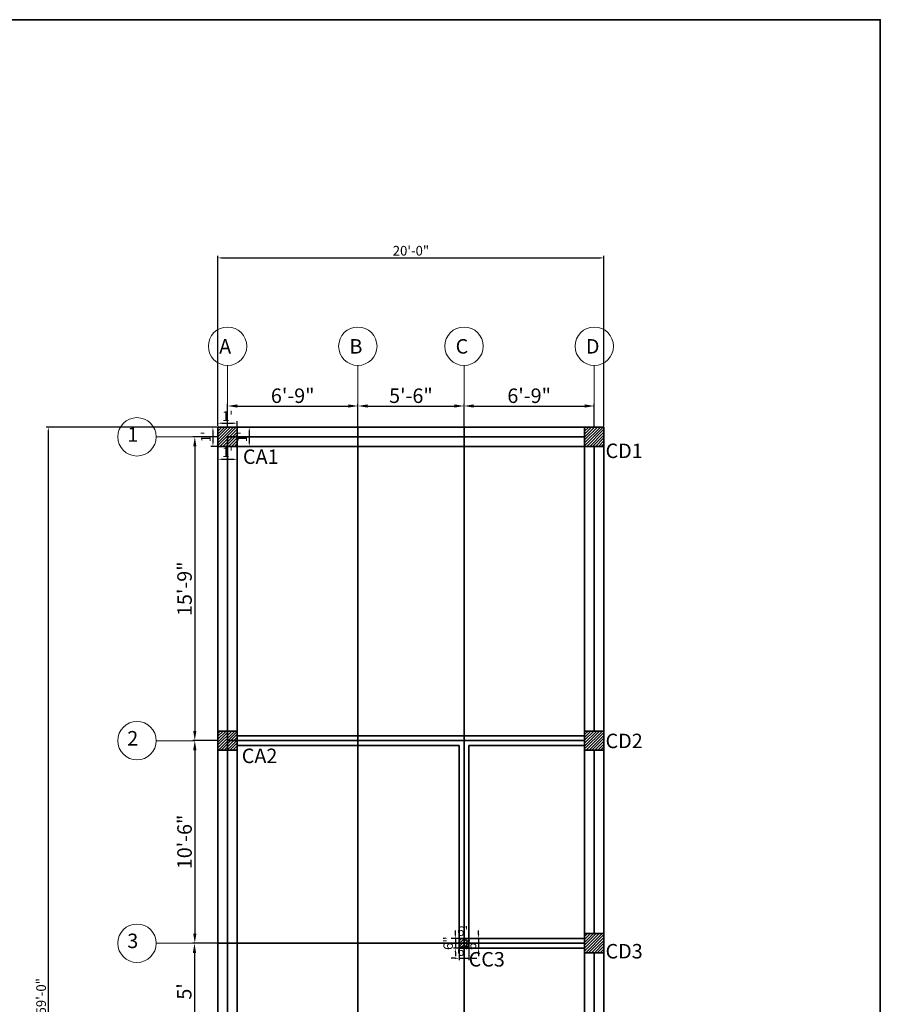
# Model space of a CAD drawing. Units: millimetres. Extents: x 20768 to 23556, y 50760 to 52704.
# Tile 36 of 36: x 23021 to 23556, y 52092 to 52704. Entities that reach past the tile are written whole.
import ezdxf

# ---------------------------------------------------------------- set-up
doc = ezdxf.new("R2010")
doc.units = ezdxf.units.MM
for name, color, linetype, lineweight in [('A-ANNO-TTLB', 7, 'Continuous', 35), ('S-ANNO-DIMS', 2, 'Continuous', 18), ('S-ANNO-TEXT', 6, 'Continuous', 18), ('S-BEAM', 3, 'Continuous', 35), ('S-COLS', 20, 'Continuous', 35), ('S-COLS-PATT', 8, 'Continuous', 13), ('S-GRID', 1, 'Continuous', 18)]:
    doc.layers.add(name, color=color, linetype=linetype, lineweight=lineweight)
doc.styles.get("Standard").update_dxf_attribs({"font": 'arial.ttf'})
doc.dimstyles.new('ISO-25', dxfattribs={"dimtxt": 6, "dimasz": 2.5, "dimexe": 1.25, "dimexo": 0.625, "dimtad": 1, "dimdec": 0, "dimlunit": 3, "dimtxsty": 'Standard', "dimcen": 2.5, "dimadec": 0, "dimazin": 0, "dimtfac": 1, "dimtdec": 0, "dimtmove": 0, "dimatfit": 3, "dimfxl": 1, "dimarcsym": 0})
pattern_1 = [(45, (1088.7427, 0), (-0.898025612, 0.898025612), [])]

# ---------------------------------------------------------------- blocks, each defined once
blk = doc.blocks.new('*D80')
at = {"layer": 'Defpoints', "color": 0, "transparency": 16777216}
for p in [(23231.01, 52463.68), (23150.01, 52450.51), (23231.01, 52450.51)]:
    blk.add_point(p, dxfattribs=at)
at = {"layer": 'S-ANNO-DIMS', "color": 0, "lineweight": -2, "transparency": 16777216}
for p, q in [((23150.01, 52451.13), (23150.01, 52464.93)), ((23231.01, 52451.13), (23231.01, 52464.93)), ((23156.01, 52463.68), (23225.01, 52463.68))]:
    blk.add_line(p, q, dxfattribs=at)
at = {"layer": 'S-ANNO-DIMS', "color": 0, "transparency": 16777216}
for points in [[(23156.01, 52464.68), (23156.01, 52462.68), (23150.01, 52463.68)], [(23225.01, 52464.68), (23225.01, 52462.68), (23231.01, 52463.68)]]:
    blk.add_solid(points, dxfattribs=at)
at = {"layer": 'S-ANNO-DIMS', "color": 0, "transparency": 16777216, "insert": (23190.51, 52468.9), "char_height": 9, "attachment_point": 5}
blk.add_mtext('6\'-9"', dxfattribs=at)
blk = doc.blocks.new('*D81')
at = {"layer": 'Defpoints', "color": 0, "transparency": 16777216}
for p in [(23297.01, 52463.68), (23231.01, 52450.51), (23297.01, 52450.51)]:
    blk.add_point(p, dxfattribs=at)
at = {"layer": 'S-ANNO-DIMS', "color": 0, "lineweight": -2, "transparency": 16777216}
for p, q in [((23231.01, 52451.13), (23231.01, 52464.93)), ((23297.01, 52451.13), (23297.01, 52464.93)), ((23237.01, 52463.68), (23291.01, 52463.68))]:
    blk.add_line(p, q, dxfattribs=at)
at = {"layer": 'S-ANNO-DIMS', "color": 0, "transparency": 16777216}
for points in [[(23237.01, 52464.68), (23237.01, 52462.68), (23231.01, 52463.68)], [(23291.01, 52464.68), (23291.01, 52462.68), (23297.01, 52463.68)]]:
    blk.add_solid(points, dxfattribs=at)
at = {"layer": 'S-ANNO-DIMS', "color": 0, "transparency": 16777216, "insert": (23264.01, 52468.9), "char_height": 9, "attachment_point": 5}
blk.add_mtext('5\'-6"', dxfattribs=at)
blk = doc.blocks.new('*D82')
at = {"layer": 'Defpoints', "color": 0, "transparency": 16777216}
for p in [(23378.01, 52463.68), (23297.01, 52450.51), (23378.01, 52450.51)]:
    blk.add_point(p, dxfattribs=at)
at = {"layer": 'S-ANNO-DIMS', "color": 0, "lineweight": -2, "transparency": 16777216}
for p, q in [((23297.01, 52451.13), (23297.01, 52464.93)), ((23378.01, 52451.13), (23378.01, 52464.93)), ((23303.01, 52463.68), (23372.01, 52463.68))]:
    blk.add_line(p, q, dxfattribs=at)
at = {"layer": 'S-ANNO-DIMS', "color": 0, "transparency": 16777216}
for points in [[(23303.01, 52464.68), (23303.01, 52462.68), (23297.01, 52463.68)], [(23372.01, 52464.68), (23372.01, 52462.68), (23378.01, 52463.68)]]:
    blk.add_solid(points, dxfattribs=at)
at = {"layer": 'S-ANNO-DIMS', "color": 0, "transparency": 16777216, "insert": (23337.51, 52468.9), "char_height": 9, "attachment_point": 5}
blk.add_mtext('6\'-9"', dxfattribs=at)
blk = doc.blocks.new('*D83')
at = {"layer": 'Defpoints', "color": 0, "transparency": 16777216}
for p in [(23144.01, 52444.51), (23129.65, 52255.51), (23144.01, 52255.51)]:
    blk.add_point(p, dxfattribs=at)
at = {"layer": 'S-ANNO-DIMS', "color": 0, "lineweight": -2, "transparency": 16777216}
for p, q in [((23143.39, 52444.51), (23128.4, 52444.51)), ((23129.65, 52438.51), (23129.65, 52261.51)), ((23143.39, 52255.51), (23128.4, 52255.51))]:
    blk.add_line(p, q, dxfattribs=at)
at = {"layer": 'S-ANNO-DIMS', "color": 0, "transparency": 16777216}
for points in [[(23128.65, 52438.51), (23130.65, 52438.51), (23129.65, 52444.51)], [(23128.65, 52261.51), (23130.65, 52261.51), (23129.65, 52255.51)]]:
    blk.add_solid(points, dxfattribs=at)
at = {"layer": 'S-ANNO-DIMS', "color": 0, "transparency": 16777216, "insert": (23124.43, 52350.01), "char_height": 9, "attachment_point": 5, "rotation": 90}
blk.add_mtext('15\'-9"', dxfattribs=at)
blk = doc.blocks.new('*D84')
at = {"layer": 'Defpoints', "color": 0, "transparency": 16777216}
for p in [(23144.01, 52255.51), (23129.65, 52129.51), (23144.01, 52129.51)]:
    blk.add_point(p, dxfattribs=at)
at = {"layer": 'S-ANNO-DIMS', "color": 0, "lineweight": -2, "transparency": 16777216}
for p, q in [((23143.39, 52255.51), (23128.4, 52255.51)), ((23129.65, 52249.51), (23129.65, 52135.51)), ((23143.39, 52129.51), (23128.4, 52129.51))]:
    blk.add_line(p, q, dxfattribs=at)
at = {"layer": 'S-ANNO-DIMS', "color": 0, "transparency": 16777216}
for points in [[(23128.65, 52249.51), (23130.65, 52249.51), (23129.65, 52255.51)], [(23128.65, 52135.51), (23130.65, 52135.51), (23129.65, 52129.51)]]:
    blk.add_solid(points, dxfattribs=at)
at = {"layer": 'S-ANNO-DIMS', "color": 0, "transparency": 16777216, "insert": (23124.43, 52192.51), "char_height": 9, "attachment_point": 5, "rotation": 90}
blk.add_mtext('10\'-6"', dxfattribs=at)
blk = doc.blocks.new('*D85')
at = {"layer": 'Defpoints', "color": 0, "transparency": 16777216}
for p in [(23144.01, 52129.51), (23129.44, 52069.51), (23144.01, 52069.51)]:
    blk.add_point(p, dxfattribs=at)
at = {"layer": 'S-ANNO-DIMS', "color": 0, "lineweight": -2, "transparency": 16777216}
for p, q in [((23143.39, 52129.51), (23128.19, 52129.51)), ((23129.44, 52123.51), (23129.44, 52075.51)), ((23143.39, 52069.51), (23128.19, 52069.51))]:
    blk.add_line(p, q, dxfattribs=at)
at = {"layer": 'S-ANNO-DIMS', "color": 0, "transparency": 16777216}
for points in [[(23128.44, 52123.51), (23130.44, 52123.51), (23129.44, 52129.51)], [(23128.44, 52075.51), (23130.44, 52075.51), (23129.44, 52069.51)]]:
    blk.add_solid(points, dxfattribs=at)
at = {"layer": 'S-ANNO-DIMS', "color": 0, "transparency": 16777216, "insert": (23124.24, 52099.51), "char_height": 9, "attachment_point": 5, "rotation": 90}
blk.add_mtext("5'", dxfattribs=at)
blk = doc.blocks.new('*D89')
at = {"layer": 'Defpoints', "color": 0, "transparency": 16777216}
for p in [(23156.01, 52452.99), (23144.01, 52450.51), (23156.01, 52450.51)]:
    blk.add_point(p, dxfattribs=at)
at = {"layer": 'S-ANNO-DIMS', "color": 0, "lineweight": -2, "transparency": 16777216}
for p, q in [((23144.01, 52451.13), (23144.01, 52454.24)), ((23146.51, 52452.99), (23153.51, 52452.99)), ((23156.01, 52451.13), (23156.01, 52454.24))]:
    blk.add_line(p, q, dxfattribs=at)
at = {"layer": 'S-ANNO-DIMS', "color": 0, "transparency": 16777216}
for points in [[(23146.51, 52453.41), (23146.51, 52452.58), (23144.01, 52452.99)], [(23153.51, 52453.41), (23153.51, 52452.58), (23156.01, 52452.99)]]:
    blk.add_solid(points, dxfattribs=at)
at = {"layer": 'S-ANNO-DIMS', "color": 0, "transparency": 16777216, "insert": (23150.01, 52456.63), "char_height": 6, "attachment_point": 5}
blk.add_mtext("1'", dxfattribs=at)
blk = doc.blocks.new('*D90')
at = {"layer": 'Defpoints', "color": 0, "transparency": 16777216}
for p in [(23156.01, 52450.51), (23156.01, 52438.51), (23163.48, 52438.51)]:
    blk.add_point(p, dxfattribs=at)
at = {"layer": 'S-ANNO-DIMS', "color": 0, "lineweight": -2, "transparency": 16777216}
for p, q in [((23156.64, 52450.51), (23164.73, 52450.51)), ((23163.48, 52448.01), (23163.48, 52441.01)), ((23156.64, 52438.51), (23164.73, 52438.51))]:
    blk.add_line(p, q, dxfattribs=at)
at = {"layer": 'S-ANNO-DIMS', "color": 0, "transparency": 16777216}
for points in [[(23163.07, 52448.01), (23163.9, 52448.01), (23163.48, 52450.51)], [(23163.07, 52441.01), (23163.9, 52441.01), (23163.48, 52438.51)]]:
    blk.add_solid(points, dxfattribs=at)
at = {"layer": 'S-ANNO-DIMS', "color": 0, "transparency": 16777216, "insert": (23159.85, 52444.51), "char_height": 6, "attachment_point": 5, "rotation": 90}
blk.add_mtext("1'", dxfattribs=at)
blk = doc.blocks.new('*D91')
at = {"layer": 'Defpoints', "color": 0, "transparency": 16777216}
for p in [(23144.01, 52438.51), (23156.01, 52438.51), (23156.01, 52430.53)]:
    blk.add_point(p, dxfattribs=at)
at = {"layer": 'S-ANNO-DIMS', "color": 0, "lineweight": -2, "transparency": 16777216}
for p, q in [((23144.01, 52437.88), (23144.01, 52429.28)), ((23156.01, 52437.88), (23156.01, 52429.28)), ((23146.51, 52430.53), (23153.51, 52430.53))]:
    blk.add_line(p, q, dxfattribs=at)
at = {"layer": 'S-ANNO-DIMS', "color": 0, "transparency": 16777216}
for points in [[(23146.51, 52430.95), (23146.51, 52430.12), (23144.01, 52430.53)], [(23153.51, 52430.95), (23153.51, 52430.12), (23156.01, 52430.53)]]:
    blk.add_solid(points, dxfattribs=at)
at = {"layer": 'S-ANNO-DIMS', "color": 0, "transparency": 16777216, "insert": (23150.01, 52434.17), "char_height": 6, "attachment_point": 5}
blk.add_mtext("1'", dxfattribs=at)
blk = doc.blocks.new('*D79')
at = {"layer": 'Defpoints', "color": 0, "transparency": 16777216}
for p in [(23144.01, 52450.51), (23140.92, 52438.51), (23144.01, 52438.51)]:
    blk.add_point(p, dxfattribs=at)
at = {"layer": 'S-ANNO-DIMS', "color": 0, "lineweight": -2, "transparency": 16777216}
for p, q in [((23143.39, 52450.51), (23139.67, 52450.51)), ((23140.92, 52448.01), (23140.92, 52441.01)), ((23143.39, 52438.51), (23139.67, 52438.51))]:
    blk.add_line(p, q, dxfattribs=at)
at = {"layer": 'S-ANNO-DIMS', "color": 0, "transparency": 16777216}
for points in [[(23140.51, 52448.01), (23141.34, 52448.01), (23140.92, 52450.51)], [(23140.51, 52441.01), (23141.34, 52441.01), (23140.92, 52438.51)]]:
    blk.add_solid(points, dxfattribs=at)
at = {"layer": 'S-ANNO-DIMS', "color": 0, "transparency": 16777216, "insert": (23137.29, 52444.51), "char_height": 6, "attachment_point": 5, "rotation": 90}
blk.add_mtext("1'", dxfattribs=at)
blk = doc.blocks.new('*D92')
at = {"layer": 'Defpoints', "color": 0, "transparency": 16777216}
for p in [(23294.01, 52132.51), (23300.01, 52132.51), (23300.01, 52132.51)]:
    blk.add_point(p, dxfattribs=at)
at = {"layer": 'S-ANNO-DIMS', "color": 0, "lineweight": -2, "transparency": 16777216}
for p, q in [((23291.51, 52132.51), (23289.01, 52132.51)), ((23294.01, 52133.13), (23294.01, 52133.76)), ((23294.01, 52132.51), (23300.01, 52132.51)), ((23300.01, 52133.13), (23300.01, 52133.76)), ((23302.51, 52132.51), (23305.01, 52132.51))]:
    blk.add_line(p, q, dxfattribs=at)
at = {"layer": 'S-ANNO-DIMS', "color": 0, "transparency": 16777216}
for points in [[(23291.51, 52132.93), (23291.51, 52132.09), (23294.01, 52132.51)], [(23302.51, 52132.93), (23302.51, 52132.09), (23300.01, 52132.51)]]:
    blk.add_solid(points, dxfattribs=at)
at = {"layer": 'S-ANNO-DIMS', "color": 0, "transparency": 16777216, "insert": (23297.01, 52136.2), "char_height": 6, "attachment_point": 5}
blk.add_mtext('6"', dxfattribs=at)
blk = doc.blocks.new('*D93')
at = {"layer": 'Defpoints', "color": 0, "transparency": 16777216}
for p in [(23300.01, 52132.51), (23300.01, 52126.51), (23306.09, 52126.51)]:
    blk.add_point(p, dxfattribs=at)
at = {"layer": 'S-ANNO-DIMS', "color": 0, "lineweight": -2, "transparency": 16777216}
for p, q in [((23306.09, 52135.01), (23306.09, 52137.51)), ((23300.64, 52132.51), (23307.34, 52132.51)), ((23306.09, 52132.51), (23306.09, 52126.51)), ((23300.64, 52126.51), (23307.34, 52126.51)), ((23306.09, 52124.01), (23306.09, 52121.51))]:
    blk.add_line(p, q, dxfattribs=at)
at = {"layer": 'S-ANNO-DIMS', "color": 0, "transparency": 16777216}
for points in [[(23305.67, 52135.01), (23306.5, 52135.01), (23306.09, 52132.51)], [(23305.67, 52124.01), (23306.5, 52124.01), (23306.09, 52126.51)]]:
    blk.add_solid(points, dxfattribs=at)
at = {"layer": 'S-ANNO-DIMS', "color": 0, "transparency": 16777216, "insert": (23302.4, 52129.51), "char_height": 6, "attachment_point": 5, "rotation": 90}
blk.add_mtext('6"', dxfattribs=at)
blk = doc.blocks.new('*D94')
at = {"layer": 'Defpoints', "color": 0, "transparency": 16777216}
for p in [(23294.01, 52126.51), (23300.01, 52126.51), (23300.01, 52120.11)]:
    blk.add_point(p, dxfattribs=at)
at = {"layer": 'S-ANNO-DIMS', "color": 0, "lineweight": -2, "transparency": 16777216}
for p, q in [((23294.01, 52125.88), (23294.01, 52118.86)), ((23300.01, 52125.88), (23300.01, 52118.86)), ((23291.51, 52120.11), (23289.01, 52120.11)), ((23294.01, 52120.11), (23300.01, 52120.11)), ((23302.51, 52120.11), (23305.01, 52120.11))]:
    blk.add_line(p, q, dxfattribs=at)
at = {"layer": 'S-ANNO-DIMS', "color": 0, "transparency": 16777216}
for points in [[(23291.51, 52120.52), (23291.51, 52119.69), (23294.01, 52120.11)], [(23302.51, 52120.52), (23302.51, 52119.69), (23300.01, 52120.11)]]:
    blk.add_solid(points, dxfattribs=at)
at = {"layer": 'S-ANNO-DIMS', "color": 0, "transparency": 16777216, "insert": (23297.01, 52123.8), "char_height": 6, "attachment_point": 5}
blk.add_mtext('6"', dxfattribs=at)
blk = doc.blocks.new('*D95')
at = {"layer": 'Defpoints', "color": 0, "transparency": 16777216}
for p in [(23294.01, 52132.51), (23291.63, 52126.51), (23294.01, 52126.51)]:
    blk.add_point(p, dxfattribs=at)
at = {"layer": 'S-ANNO-DIMS', "color": 0, "lineweight": -2, "transparency": 16777216}
for p, q in [((23291.63, 52135.01), (23291.63, 52137.51)), ((23293.39, 52132.51), (23290.38, 52132.51)), ((23291.63, 52132.51), (23291.63, 52126.51)), ((23293.39, 52126.51), (23290.38, 52126.51)), ((23291.63, 52124.01), (23291.63, 52121.51))]:
    blk.add_line(p, q, dxfattribs=at)
at = {"layer": 'S-ANNO-DIMS', "color": 0, "transparency": 16777216}
for points in [[(23291.21, 52135.01), (23292.04, 52135.01), (23291.63, 52132.51)], [(23291.21, 52124.01), (23292.04, 52124.01), (23291.63, 52126.51)]]:
    blk.add_solid(points, dxfattribs=at)
at = {"layer": 'S-ANNO-DIMS', "color": 0, "transparency": 16777216, "insert": (23287.94, 52129.51), "char_height": 6, "attachment_point": 5, "rotation": 90}
blk.add_mtext('6"', dxfattribs=at)
blk = doc.blocks.new('GRID-BUBBLE')
blk.add_line((47.87, 11.93), (23.87, 11.93))
blk.add_circle((11.93, 11.93), 11.93)
blk = doc.blocks.new('*D227')
at = {"layer": 'Defpoints', "color": 0, "transparency": 16777216}
for p in [(23384.01, 52555.8), (23144.01, 52450.51), (23384.01, 52450.51)]:
    blk.add_point(p, dxfattribs=at)
at = {"layer": 'S-ANNO-DIMS', "color": 0, "lineweight": -2, "transparency": 16777216}
for p, q in [((23144.01, 52451.13), (23144.01, 52557.05)), ((23384.01, 52451.13), (23384.01, 52557.05)), ((23146.51, 52555.8), (23381.51, 52555.8))]:
    blk.add_line(p, q, dxfattribs=at)
at = {"layer": 'S-ANNO-DIMS', "color": 0, "transparency": 16777216}
for points in [[(23146.51, 52556.22), (23146.51, 52555.38), (23144.01, 52555.8)], [(23381.51, 52556.22), (23381.51, 52555.38), (23384.01, 52555.8)]]:
    blk.add_solid(points, dxfattribs=at)
at = {"layer": 'S-ANNO-DIMS', "color": 0, "transparency": 16777216, "insert": (23264.01, 52559.49), "char_height": 6, "attachment_point": 5}
blk.add_mtext('20\'-0"', dxfattribs=at)
blk = doc.blocks.new('*D228')
at = {"layer": 'Defpoints', "color": 0, "transparency": 16777216}
for p in [(23144.01, 52450.51), (23038.57, 51742.51), (23144.01, 51742.51)]:
    blk.add_point(p, dxfattribs=at)
at = {"layer": 'S-ANNO-DIMS', "color": 0, "lineweight": -2, "transparency": 16777216}
for p, q in [((23143.39, 52450.51), (23037.32, 52450.51)), ((23038.57, 52448.01), (23038.57, 51745.01)), ((23143.39, 51742.51), (23037.32, 51742.51))]:
    blk.add_line(p, q, dxfattribs=at)
at = {"layer": 'S-ANNO-DIMS', "color": 0, "transparency": 16777216}
for points in [[(23038.16, 52448.01), (23038.99, 52448.01), (23038.57, 52450.51)], [(23038.16, 51745.01), (23038.99, 51745.01), (23038.57, 51742.51)]]:
    blk.add_solid(points, dxfattribs=at)
at = {"layer": 'S-ANNO-DIMS', "color": 0, "transparency": 16777216, "insert": (23034.88, 52096.51), "char_height": 6, "attachment_point": 5, "rotation": 90}
blk.add_mtext('59\'-0"', dxfattribs=at)

msp = doc.modelspace()

# ---------------------------------------------------------------- hatches: boundary and pattern name
at = {"layer": 'S-COLS-PATT'}
h = msp.add_hatch(dxfattribs=at)
h.set_pattern_fill('ANSI31', color=256, scale=0.4)
h.set_pattern_definition(pattern_1)
h.paths.add_polyline_path([(23156.01, 52450.51), (23144.01, 52450.51), (23144.01, 52438.51), (23150.01, 52438.51), (23150.01, 52444.51), (23156.01, 52444.51)])
h = msp.add_hatch(dxfattribs=at)
h.set_pattern_fill('ANSI31', color=256, scale=0.4)
h.set_pattern_definition(pattern_1)
h.paths.add_polyline_path([(23384.01, 52450.51), (23372.01, 52450.51), (23372.01, 52438.51), (23384.01, 52438.51)])
h = msp.add_hatch(dxfattribs=at)
h.set_pattern_fill('ANSI31', color=256, scale=0.4)
h.set_pattern_definition(pattern_1)
h.paths.add_polyline_path([(23156.01, 52444.51), (23150.01, 52444.51), (23150.01, 52438.51), (23156.01, 52438.51)], flags=17)
h = msp.add_hatch(dxfattribs=at)
h.set_pattern_fill('ANSI31', color=256, scale=0.4)
h.set_pattern_definition([(45, (861.8838, 0), (-0.898025612, 0.898025612), [])])
h.paths.add_polyline_path([(23156.01, 52261.51), (23144.01, 52261.51), (23144.01, 52249.51), (23156.01, 52249.51)])
h = msp.add_hatch(dxfattribs=at)
h.set_pattern_fill('ANSI31', color=256, scale=0.4)
h.set_pattern_definition(pattern_1)
h.paths.add_polyline_path([(23384.01, 52261.51), (23372.01, 52261.51), (23372.01, 52249.51), (23384.01, 52249.51)])
h = msp.add_hatch(dxfattribs=at)
h.set_pattern_fill('ANSI31', color=256, scale=0.4)
h.set_pattern_definition(pattern_1)
h.paths.add_polyline_path([(23384.01, 52135.51), (23372.01, 52135.51), (23372.01, 52123.51), (23384.01, 52123.51)])
h = msp.add_hatch(dxfattribs=at)
h.set_pattern_fill('ANSI31', color=256, scale=0.4)
h.set_pattern_definition(pattern_1)
h.paths.add_polyline_path([(23297.01, 52132.51), (23294.01, 52132.51), (23294.01, 52129.51), (23297.01, 52129.51)])
h = msp.add_hatch(dxfattribs=at)
h.set_pattern_fill('ANSI31', color=256, scale=0.4)
h.set_pattern_definition(pattern_1)
h.paths.add_polyline_path([(23297.01, 52129.51), (23294.01, 52129.51), (23294.01, 52126.51), (23297.01, 52126.51)], flags=17)
h = msp.add_hatch(dxfattribs=at)
h.set_pattern_fill('ANSI31', color=256, scale=0.4)
h.set_pattern_definition(pattern_1)
h.paths.add_polyline_path([(23300.01, 52132.51), (23297.01, 52132.51), (23297.01, 52129.51), (23300.01, 52129.51)])
h = msp.add_hatch(dxfattribs=at)
h.set_pattern_fill('ANSI31', color=256, scale=0.4)
h.set_pattern_definition(pattern_1)
h.paths.add_polyline_path([(23300.01, 52129.51), (23297.01, 52129.51), (23297.01, 52126.51), (23300.01, 52126.51)])

# ---------------------------------------------------------------- linework, layer by layer
at = {"layer": 'A-ANNO-TTLB'}
msp.add_lwpolyline([(20768.14, 52703.98), (23555.8, 52703.98), (23555.8, 51623.53), (20768.14, 51623.53)], close=True, dxfattribs=at)
at = {"layer": 'S-BEAM'}
for p, q in [((23144.01, 52450.51), (23384.01, 52450.51)), ((23144.01, 52450.51), (23144.01, 51742.51)), ((23156.01, 52450.51), (23156.01, 51742.51)), ((23231.01, 52450.51), (23231.01, 51748.51)), ((23297.01, 52450.51), (23297.01, 51748.51)), ((23372.01, 52450.51), (23372.01, 51742.51)), ((23384.01, 52450.51), (23384.01, 51742.51)), ((23150.01, 52444.51), (23150.01, 51742.51)), ((23150.01, 52444.51), (23372.01, 52444.51)), ((23144.01, 52438.51), (23384.01, 52438.51)), ((23378.01, 52438.51), (23378.01, 52261.51)), ((23156.01, 52258.51), (23297.01, 52258.51)), ((23297.01, 52258.51), (23372.01, 52258.51)), ((23150.01, 52255.51), (23372.01, 52255.51)), ((23156.01, 52252.51), (23294.01, 52252.51)), ((23294.01, 52252.51), (23294.01, 52126.51)), ((23300.01, 52252.51), (23300.01, 52126.51)), ((23300.01, 52252.51), (23372.01, 52252.51)), ((23378.01, 52249.51), (23378.01, 52135.51)), ((23144.01, 52129.51), (23372.01, 52129.51)), ((23294.01, 52132.51), (23372.01, 52132.51)), ((23294.01, 52126.51), (23372.01, 52126.51)), ((23378.01, 52123.51), (23378.01, 51823.51))]:
    msp.add_line(p, q, dxfattribs=at)
at = {"layer": 'S-COLS'}
for points in [[(23144.01, 52450.51), (23156.01, 52450.51), (23156.01, 52438.51), (23144.01, 52438.51)], [(23372.01, 52450.51), (23384.01, 52450.51), (23384.01, 52438.51), (23372.01, 52438.51)], [(23156.01, 52261.51), (23144.01, 52261.51), (23144.01, 52249.51), (23156.01, 52249.51)], [(23372.01, 52261.51), (23384.01, 52261.51), (23384.01, 52249.51), (23372.01, 52249.51)], [(23372.01, 52135.51), (23384.01, 52135.51), (23384.01, 52123.51), (23372.01, 52123.51)], [(23300.01, 52132.51), (23294.01, 52132.51), (23294.01, 52126.51), (23300.01, 52126.51)]]:
    msp.add_lwpolyline(points, close=True, dxfattribs=at)
at = {"layer": 'S-GRID'}
for p, q in [((23150.01, 52464.93), (23150.01, 52488.93)), ((23231.01, 52464.93), (23231.01, 52488.93)), ((23297.01, 52464.93), (23297.01, 52488.93)), ((23378.01, 52464.93), (23378.01, 52488.93))]:
    msp.add_line(p, q, dxfattribs=at)
for centre in [(23150.01, 52500.87), (23231.01, 52500.87), (23297.01, 52500.87), (23378.01, 52500.87)]:
    msp.add_circle(centre, 11.93, dxfattribs=at)

# ---------------------------------------------------------------- block references
for p in [(23081.78, 52432.57), (23081.78, 52243.57), (23081.78, 52117.57)]:
    msp.add_blockref('GRID-BUBBLE', p, dxfattribs=at)

# ---------------------------------------------------------------- texts
at = {"layer": 'S-ANNO-TEXT', "char_height": 9, "attachment_point": 1}
for s, width, insert in [('  A', 27.5349, (23139.29, 52505.28)), ('  B', 27.5349, (23220.29, 52505.28)), ('  C', 27.5349, (23286.29, 52505.28)), ('  D', 27.5349, (23367.29, 52505.28)), ('  1', 27.5349, (23082.17, 52450.48)), ('CD1', 38.9452, (23385.01, 52440.29)), ('CA1', 15.3341, (23159.58, 52436.64)), ('  2', 27.5349, (23082.17, 52261.48)), ('CD2', 15.3341, (23385.01, 52259.84)), ('CA2', 15.3341, (23158.84, 52250.57)), ('  3', 27.5349, (23082.17, 52135.48)), ('CD3', 15.3341, (23385.01, 52129.03)), ('CC3', 15.3341, (23299.9, 52124))]:
    msp.add_mtext_dynamic_manual_height_columns(s, width=width, gutter_width=12.5, heights=[0], dxfattribs=dict(at, insert=insert))

# ---------------------------------------------------------------- dimensions: what is measured, and where the dimension line sits
at = {"layer": 'S-ANNO-DIMS'}
for base, p1, p2, override, picture, middle in [((23384.01, 52555.8), (23144.01, 52450.51), (23384.01, 52450.51), {"dimdec": 1, "dimlfac": 1, "dimrnd": 0, "dimzin": 1, "dimdsep": 46, "dimlunit": 4, "dimfrac": 2}, '*D227', (23264.01, 52559.49)), ((23231.01, 52463.68), (23150.01, 52450.51), (23231.01, 52450.51), {"dimtxt": 9, "dimasz": 6, "dimclrd": 0, "dimclre": 0, "dimclrt": 0}, '*D80', (23190.51, 52468.9)), ((23297.01, 52463.68), (23231.01, 52450.51), (23297.01, 52450.51), {"dimtxt": 9, "dimasz": 6, "dimclrd": 0, "dimclre": 0, "dimclrt": 0}, '*D81', (23264.01, 52468.9)), ((23378.01, 52463.68), (23297.01, 52450.51), (23378.01, 52450.51), {"dimtxt": 9, "dimasz": 6, "dimclrd": 0, "dimclre": 0, "dimclrt": 0}, '*D82', (23337.51, 52468.9)), ((23156.01, 52452.99), (23144.01, 52450.51), (23156.01, 52450.51), {"dimclrd": 0, "dimclre": 0, "dimclrt": 0}, '*D89', (23150.01, 52456.63)), ((23156.01, 52430.53), (23144.01, 52438.51), (23156.01, 52438.51), {"dimclrd": 0, "dimclre": 0, "dimclrt": 0}, '*D91', (23150.01, 52434.17))]:
    dim = msp.add_linear_dim(base=base, p1=p1, p2=p2, dimstyle='ISO-25', override=override, dxfattribs=at)
    dim.commit()
    dim.dimension.update_dxf_attribs({"geometry": picture, "text_midpoint": middle})
for base, p1, p2, override, picture, middle in [((23038.57, 51742.51), (23144.01, 52450.51), (23144.01, 51742.51), {"dimdec": 1, "dimlfac": 1, "dimrnd": 0, "dimzin": 1, "dimdsep": 46, "dimlunit": 4, "dimfrac": 2}, '*D228', (23034.88, 52096.51)), ((23140.92, 52438.51), (23144.01, 52450.51), (23144.01, 52438.51), {"dimclrd": 0, "dimclre": 0, "dimclrt": 0}, '*D79', (23137.29, 52444.51)), ((23163.48, 52438.51), (23156.01, 52450.51), (23156.01, 52438.51), {"dimclrd": 0, "dimclre": 0, "dimclrt": 0}, '*D90', (23159.85, 52444.51)), ((23129.65, 52255.51), (23144.01, 52444.51), (23144.01, 52255.51), {"dimtxt": 9, "dimasz": 6, "dimclrd": 0, "dimclre": 0, "dimclrt": 0}, '*D83', (23124.43, 52350.01)), ((23129.65, 52129.51), (23144.01, 52255.51), (23144.01, 52129.51), {"dimtxt": 9, "dimasz": 6, "dimclrd": 0, "dimclre": 0, "dimclrt": 0}, '*D84', (23124.43, 52192.51)), ((23129.44, 52069.51), (23144.01, 52129.51), (23144.01, 52069.51), {"dimtxt": 9, "dimasz": 6, "dimclrd": 0, "dimclre": 0, "dimclrt": 0}, '*D85', (23124.24, 52099.51))]:
    dim = msp.add_linear_dim(base=base, p1=p1, p2=p2, angle=90, dimstyle='ISO-25', override=override, dxfattribs=at)
    dim.commit()
    dim.dimension.update_dxf_attribs({"geometry": picture, "text_midpoint": middle})
for base, p1, p2, picture, middle in [((23300.01, 52132.51), (23294.01, 52132.51), (23300.01, 52132.51), '*D92', (23297.01, 52132.51)), ((23300.01, 52120.11), (23294.01, 52126.51), (23300.01, 52126.51), '*D94', (23297.01, 52120.11))]:
    dim = msp.add_linear_dim(base=base, p1=p1, p2=p2, dimstyle='ISO-25', override={"dimclrd": 0, "dimclre": 0, "dimclrt": 0}, dxfattribs=at)
    dim.commit()
    dim.dimension.update_dxf_attribs({"geometry": picture, "text_midpoint": middle, "dimtype": 160})
for base, p1, p2, picture, middle in [((23291.63, 52126.51), (23294.01, 52132.51), (23294.01, 52126.51), '*D95', (23291.63, 52129.51)), ((23306.09, 52126.51), (23300.01, 52132.51), (23300.01, 52126.51), '*D93', (23306.09, 52129.51))]:
    dim = msp.add_linear_dim(base=base, p1=p1, p2=p2, angle=90, dimstyle='ISO-25', override={"dimclrd": 0, "dimclre": 0, "dimclrt": 0}, dxfattribs=at)
    dim.commit()
    dim.dimension.update_dxf_attribs({"geometry": picture, "text_midpoint": middle, "dimtype": 160})

doc.saveas('drawing.dxf')
